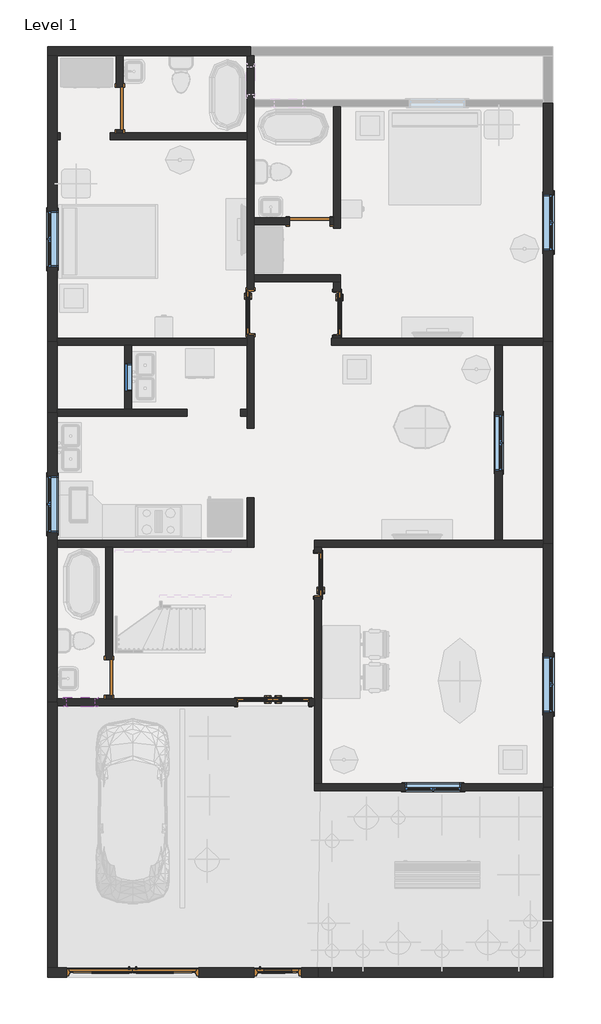
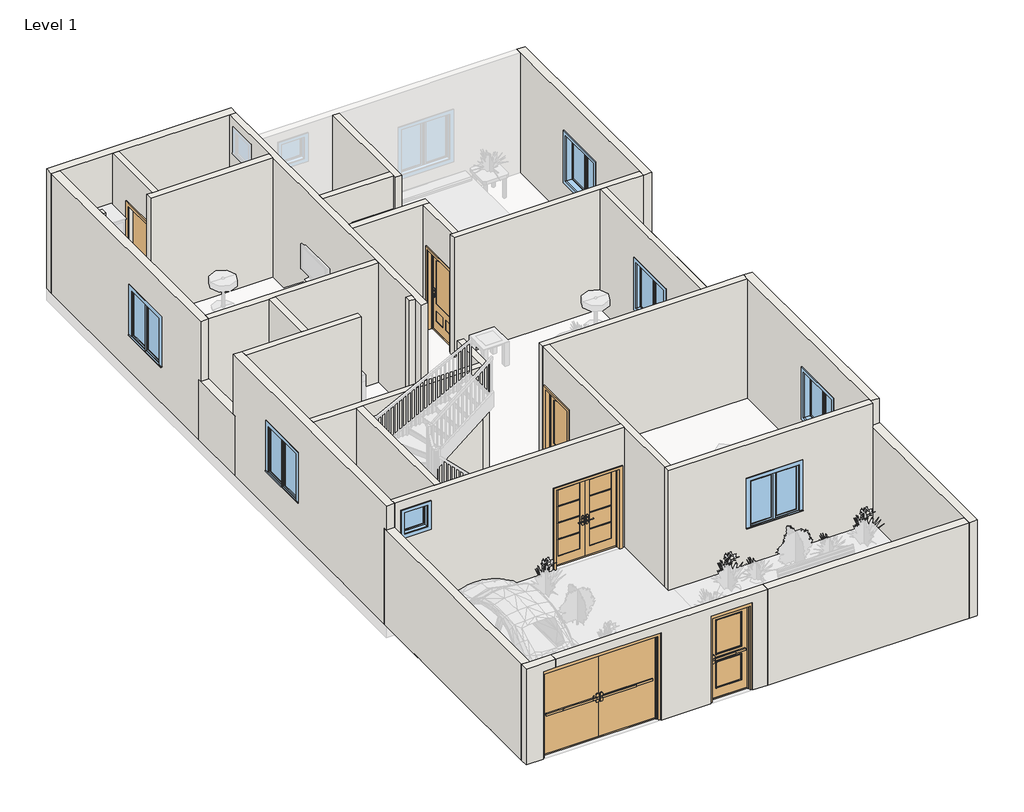
# One storey, part 1 of 3: 33 walls, 9 doors, 8 windows.
"""IFC4 building model written with IfcOpenShell, lengths in millimetres."""

from ifc_helpers import new_model, si_unit, frame, origin, origin_with_axes, place, context, project, spatial, polyline, outline, extrude, faceted_brep, transform, mapped, element, save
from components import door_808aeb8e, door_5d363d20, door_b5c84c7e, door_94998e6c, door_exterior_single_two_lite_door_exterior_single_two_lite_36a17ea7, door_059fdd7e, door_b6e9fca3, door_16372e1c, window_0862ab64, window_be30da88, window_aff1bc2a, window_3d781103

model = new_model("IFC4")

# Units and contexts
model_context = context("Model", 3, world=origin())
ifc_project = project(units=[si_unit("LENGTHUNIT", "METRE", prefix="MILLI")], contexts=[model_context])

# Site, building, storey
site = spatial("IfcSite", under=ifc_project)
building = spatial("IfcBuilding", under=site)
storey = spatial("IfcBuildingStorey", under=building, Name="Level 1", Elevation=0.0)

# Doors
placement = place(None, origin())
door_shape = door_808aeb8e(model_context)
element("IfcDoor", 1, ObjectType="36\" x 80\"", at=placement, inside=storey, context=model_context, shape_type="MappedRepresentation", body=[
    mapped(door_shape, transform((-7436.4726606, 8433.499435, 0.0), x_axis=(0.0, 1.0, 0.0), y_axis=(-1.0, 0.0, 0.0), z_axis=(0.0, 0.0, 1.0))),
])
element("IfcDoor", 2, ObjectType="36\" x 80\"", at=placement, inside=storey, context=model_context, shape_type="MappedRepresentation", body=[
    mapped(door_shape, transform((-5982.3226606, 2794.699435, 0.0), x_axis=(0.0, -1.0, 0.0), y_axis=(1.0, 0.0, 0.0), z_axis=(0.0, 0.0, 1.0))),
])
door_2_shape = door_5d363d20(model_context)
element("IfcDoor", 3, ObjectType="36\" x 80\"", at=placement, inside=storey, context=model_context, shape_type="MappedRepresentation", body=[
    mapped(door_2_shape, transform((-5575.9226606, 8408.099435, 0.0), x_axis=(0.0, 1.0, 0.0), y_axis=(-1.0, 0.0, 0.0), z_axis=(0.0, 0.0, 1.0))),
])
door_3_shape = door_b5c84c7e(model_context)
element("IfcDoor", 4, ObjectType="Door-Exterior-Double : 108\" x 84\"", at=placement, inside=storey, context=model_context, shape_type="MappedRepresentation", body=[
    mapped(door_3_shape, transform((-9973.2976606, -5771.450565, 0.0), x_axis=(1.0, 0.0, 0.0), y_axis=(0.0, 1.0, 0.0), z_axis=(0.0, 0.0, 1.0))),
])
door_4_shape = door_94998e6c(model_context)
element("IfcDoor", 5, ObjectType="Door-Exterior-Double-Full Glass-Wood_Clad : 60\" x 80\"", at=placement, inside=storey, context=model_context, shape_type="MappedRepresentation", body=[
    mapped(door_4_shape, transform((-6950.6976606, 54.674435, 0.0), x_axis=(1.0, 0.0, 0.0), y_axis=(0.0, 1.0, 0.0), z_axis=(0.0, 0.0, 1.0))),
])
door_exterior_single_two_lite_door_exterior_single_two_lite_shape = door_exterior_single_two_lite_door_exterior_single_two_lite_36a17ea7(model_context)
element("IfcDoor", 6, ObjectType="Door-Exterior-Single-Two_Lite : Door-Exterior-Single-Two_Lite", at=placement, inside=storey, context=model_context, shape_type="MappedRepresentation", body=[
    mapped(door_exterior_single_two_lite_door_exterior_single_two_lite_shape, transform((-6849.0976606, -5771.450565, 0.0), x_axis=(1.0, 0.0, 0.0), y_axis=(0.0, 1.0, 0.0), z_axis=(0.0, 0.0, 1.0))),
])
door_5_shape = door_059fdd7e(model_context)
element("IfcDoor", 7, ObjectType="Single-Flush : 30\" x 80\"", at=placement, inside=storey, context=model_context, shape_type="MappedRepresentation", body=[
    mapped(door_5_shape, transform((-10481.2976606, 584.899435, 0.0), x_axis=(0.0, -1.0, 0.0), y_axis=(1.0, 0.0, 0.0), z_axis=(0.0, 0.0, 1.0))),
])
door_6_shape = door_b6e9fca3(model_context)
element("IfcDoor", 8, ObjectType="Single-Flush : 34\" x 84\"", at=placement, inside=storey, context=model_context, shape_type="MappedRepresentation", body=[
    mapped(door_6_shape, transform((-6163.2976606, 10389.299435, 0.0), x_axis=(1.0, 0.0, 0.0), y_axis=(0.0, 1.0, 0.0), z_axis=(0.0, 0.0, 1.0))),
])
door_7_shape = door_16372e1c(model_context)
element("IfcDoor", 9, ObjectType="Single-Flush : 36\" x 84\"", at=placement, inside=storey, context=model_context, shape_type="MappedRepresentation", body=[
    mapped(door_7_shape, transform((-10252.6976606, 12814.999435, 0.0), x_axis=(0.0, -1.0, 0.0), y_axis=(1.0, 0.0, 0.0), z_axis=(0.0, 0.0, 1.0))),
])

# Walls
element("IfcWall", 10, at=placement, inside=storey, context=model_context, shape_type="SweptSolid", body=[
    extrude(outline(polyline([(-5985.4976606, -5663.500565), (-1134.0976606, -5663.500565), (-1134.0976606, -5866.700565), (-5985.4976606, -5866.700565), (-5985.4976606, -5663.500565)])), origin_with_axes(), (0.0, 0.0, 1.0), 2438.4),
])
element("IfcWall", 11, at=placement, inside=storey, context=model_context, shape_type="Brep", body=[
    faceted_brep([(-11598.8976606, -5663.500565, 0.0), (-11598.8976606, -24.700565, 0.0), (-11598.8976606, 51.499435, 0.0), (-11598.8976606, 51.499435, 2438.4), (-11598.8976606, -5663.500565, 2438.4), (-11802.0976606, -5663.500565, 0.0), (-11802.0976606, -5663.500565, 2438.4), (-11802.0976606, 51.499435, 2438.4), (-11802.0976606, 51.499435, 0.0)], [[[0, 1, 2, 3, 4]], [[5, 6, 7, 8]], [[2, 1, 0, 5, 8]], [[3, 2, 8, 7]], [[4, 3, 7, 6]], [[0, 4, 6, 5]]]),
])
element("IfcWall", 12, at=placement, inside=storey, context=model_context, shape_type="SweptSolid", body=[
    extrude(outline(polyline([(2438.4, -5985.4976606), (2438.4, -11090.8976606), (2235.2, -11090.8976606), (2235.2, -8550.8976606), (0.0, -8550.8976606), (0.0, -7357.0976606), (2235.2, -7357.0976606), (2235.2, -6341.0976606), (0.0, -6341.0976606), (0.0, -5985.4976606), (2438.4, -5985.4976606)])), frame((0.0, -5866.700565, 0.0), z_axis=(0.0, 1.0, 0.0), x_axis=(0.0, 0.0, 1.0)), (0.0, 0.0, 1.0), 203.2),
])
element("IfcWall", 13, at=placement, inside=storey, context=model_context, shape_type="Brep", body=[
    faceted_brep([(-1134.0976606, -1790.000565, 0.0), (-1134.0976606, -1853.500565, 0.0), (-1134.0976606, -5663.500565, 0.0), (-1134.0976606, -5866.700565, 0.0), (-1134.0976606, -5866.700565, 2438.4), (-1134.0976606, -5663.500565, 2438.4), (-1134.0976606, -1790.000565, 2438.4), (-930.8976606, -1790.000565, 0.0), (-930.8976606, -1790.000565, 2438.4), (-930.8976606, -5866.700565, 2438.4), (-930.8976606, -5866.700565, 0.0)], [[[0, 1, 2, 3, 4, 5, 6]], [[7, 8, 9, 10]], [[3, 2, 1, 0, 7, 10]], [[6, 5, 4, 9, 8]], [[0, 6, 8, 7]], [[4, 3, 10, 9]]]),
])
element("IfcWall", 14, at=placement, inside=storey, context=model_context, shape_type="Brep", body=[
    faceted_brep([(-11802.0976606, -5663.500565, 2438.4), (-11598.8976606, -5663.500565, 2438.4), (-11090.8976606, -5663.500565, 2438.4), (-11090.8976606, -5663.500565, 2235.2), (-11395.6976606, -5663.500565, 2235.2), (-11395.6976606, -5663.500565, 0.0), (-11598.8976606, -5663.500565, 0.0), (-11802.0976606, -5663.500565, 0.0), (-11090.8976606, -5866.700565, 2438.4), (-11802.0976606, -5866.700565, 2438.4), (-11802.0976606, -5866.700565, 0.0), (-11395.6976606, -5866.700565, 0.0), (-11395.6976606, -5866.700565, 2235.2), (-11090.8976606, -5866.700565, 2235.2)], [[[0, 1, 2, 3, 4, 5, 6, 7]], [[8, 9, 10, 11, 12, 13]], [[10, 7, 6, 5, 11]], [[2, 1, 0, 9, 8]], [[2, 8, 13, 3]], [[0, 7, 10, 9]], [[12, 4, 3, 13]], [[4, 12, 11, 5]]]),
])
element("IfcWall", 15, ObjectType="Generic - 8\"", at=placement, inside=storey, context=model_context, shape_type="Brep", body=[
    faceted_brep([(-11802.0976606, 13945.299435, 0.0), (-11598.8976606, 13945.299435, 0.0), (-10328.8976606, 13945.299435, 0.0), (-10176.4976606, 13945.299435, 0.0), (-7509.4976606, 13945.299435, 0.0), (-7433.2976606, 13945.299435, 0.0), (-7433.2976606, 13945.299435, 1524.0), (-7357.0976606, 13945.299435, 1524.0), (-7357.0976606, 13945.299435, 3048.0), (-7509.4976606, 13945.299435, 3048.0), (-10176.4976606, 13945.299435, 3048.0), (-10328.8976606, 13945.299435, 3048.0), (-11598.8976606, 13945.299435, 3048.0), (-11802.0976606, 13945.299435, 3048.0), (-11802.0976606, 14148.499435, 0.0), (-11802.0976606, 14148.499435, 3048.0), (-7357.0976606, 14148.499435, 3048.0), (-7357.0976606, 14148.499435, 1524.0), (-7433.2976606, 14148.499435, 1524.0), (-7433.2976606, 14148.499435, 0.0)], [[[0, 1, 2, 3, 4, 5, 6, 7, 8, 9, 10, 11, 12, 13]], [[14, 15, 16, 17, 18, 19]], [[5, 4, 3, 2, 1, 0, 14, 19]], [[0, 13, 15, 14]], [[6, 5, 19, 18]], [[17, 7, 6, 18]], [[8, 7, 17, 16]], [[13, 12, 11, 10, 9, 8, 16, 15]]]),
])
element("IfcWall", 16, ObjectType="Generic - 8\"", at=placement, inside=storey, context=model_context, shape_type="Brep", body=[
    faceted_brep([(-1134.0976606, 7798.499435, 0.0), (-1134.0976606, 7722.299435, 0.0), (-1134.0976606, 3531.299435, 0.0), (-1134.0976606, 3455.099435, 0.0), (-1134.0976606, 3455.099435, 1524.0), (-1134.0976606, 3531.299435, 1524.0), (-1134.0976606, 7722.299435, 1524.0), (-1134.0976606, 7798.499435, 1524.0), (-930.8976606, 7798.499435, 0.0), (-930.8976606, 7798.499435, 1524.0), (-930.8976606, 7722.299435, 1524.0), (-930.8976606, 3531.299435, 1524.0), (-930.8976606, 3455.099435, 1524.0), (-930.8976606, 3455.099435, 0.0)], [[[0, 1, 2, 3, 4, 5, 6, 7]], [[8, 9, 10, 11, 12, 13]], [[3, 2, 1, 0, 8, 13]], [[4, 3, 13, 12]], [[7, 6, 5, 4, 12, 11, 10, 9]], [[0, 7, 9, 8]]]),
])
element("IfcWall", 17, ObjectType="Generic - 8\"", at=placement, inside=storey, context=model_context, shape_type="Brep", body=[
    faceted_brep([(-1134.0976606, 3455.099435, 0.0), (-1134.0976606, 3378.899435, 0.0), (-1134.0976606, -1764.600565, 0.0), (-1134.0976606, -1764.600565, 3048.0), (-1134.0976606, 3378.899435, 3048.0), (-1134.0976606, 3531.299435, 3048.0), (-1134.0976606, 3531.299435, 1524.0), (-1134.0976606, 3455.099435, 1524.0), (-1134.0976606, -177.100565, 2133.6), (-1134.0976606, -177.100565, 914.4), (-1134.0976606, 1042.099435, 914.4), (-1134.0976606, 1042.099435, 2133.6), (-930.8976606, 3455.099435, 0.0), (-930.8976606, 3455.099435, 1524.0), (-930.8976606, 3531.299435, 1524.0), (-930.8976606, 3531.299435, 3048.0), (-930.8976606, -1764.600565, 3048.0), (-930.8976606, -1764.600565, 0.0), (-930.8976606, -177.100565, 2133.6), (-930.8976606, 1042.099435, 2133.6), (-930.8976606, 1042.099435, 914.4), (-930.8976606, -177.100565, 914.4)], [[[0, 1, 2, 3, 4, 5, 6, 7], [8, 9, 10, 11]], [[12, 13, 14, 15, 16, 17], [18, 19, 20, 21]], [[2, 1, 0, 12, 17]], [[3, 2, 17, 16]], [[0, 7, 13, 12]], [[6, 14, 13, 7]], [[6, 5, 15, 14]], [[9, 8, 18, 21]], [[10, 9, 21, 20]], [[11, 10, 20, 19]], [[8, 11, 19, 18]], [[5, 4, 3, 16, 15]]]),
])
element("IfcWall", 18, ObjectType="Generic - 8\"", at=placement, inside=storey, context=model_context, shape_type="Brep", body=[
    faceted_brep([(-1134.0976606, 12929.299435, 0.0), (-1134.0976606, 12853.099435, 0.0), (-1134.0976606, 7874.699435, 0.0), (-1134.0976606, 7798.499435, 0.0), (-1134.0976606, 7798.499435, 1524.0), (-1134.0976606, 7722.299435, 1524.0), (-1134.0976606, 7722.299435, 3048.0), (-1134.0976606, 7874.699435, 3048.0), (-1134.0976606, 12853.099435, 3048.0), (-1134.0976606, 13005.499435, 3048.0), (-1134.0976606, 13005.499435, 1524.0), (-1134.0976606, 12929.299435, 1524.0), (-1134.0976606, 9754.299435, 2133.6), (-1134.0976606, 9754.299435, 914.4), (-1134.0976606, 10973.499435, 914.4), (-1134.0976606, 10973.499435, 2133.6), (-930.8976606, 12929.299435, 0.0), (-930.8976606, 12929.299435, 1524.0), (-930.8976606, 13005.499435, 1524.0), (-930.8976606, 13005.499435, 3048.0), (-930.8976606, 7722.299435, 3048.0), (-930.8976606, 7722.299435, 1524.0), (-930.8976606, 7798.499435, 1524.0), (-930.8976606, 7798.499435, 0.0), (-930.8976606, 9754.299435, 2133.6), (-930.8976606, 10973.499435, 2133.6), (-930.8976606, 10973.499435, 914.4), (-930.8976606, 9754.299435, 914.4)], [[[0, 1, 2, 3, 4, 5, 6, 7, 8, 9, 10, 11], [12, 13, 14, 15]], [[16, 17, 18, 19, 20, 21, 22, 23], [24, 25, 26, 27]], [[3, 2, 1, 0, 16, 23]], [[4, 3, 23, 22]], [[21, 5, 4, 22]], [[6, 5, 21, 20]], [[0, 11, 17, 16]], [[10, 18, 17, 11]], [[10, 9, 19, 18]], [[13, 12, 24, 27]], [[14, 13, 27, 26]], [[15, 14, 26, 25]], [[12, 15, 25, 24]], [[9, 8, 7, 6, 20, 19]]]),
])
element("IfcWall", 19, ObjectType="Generic - 8\"", at=placement, inside=storey, context=model_context, shape_type="Brep", body=[
    faceted_brep([(-11598.8976606, 7798.499435, 0.0), (-11598.8976606, 7874.699435, 0.0), (-11598.8976606, 12141.899435, 0.0), (-11598.8976606, 12294.299435, 0.0), (-11598.8976606, 13945.299435, 0.0), (-11598.8976606, 13945.299435, 3048.0), (-11598.8976606, 12294.299435, 3048.0), (-11598.8976606, 12141.899435, 3048.0), (-11598.8976606, 7874.699435, 3048.0), (-11598.8976606, 7722.299435, 3048.0), (-11598.8976606, 7722.299435, 1524.0), (-11598.8976606, 7798.499435, 1524.0), (-11598.8976606, 10617.899435, 2133.6), (-11598.8976606, 10617.899435, 914.4), (-11598.8976606, 9398.699435, 914.4), (-11598.8976606, 9398.699435, 2133.6), (-11802.0976606, 7798.499435, 0.0), (-11802.0976606, 7798.499435, 1524.0), (-11802.0976606, 7722.299435, 1524.0), (-11802.0976606, 7722.299435, 3048.0), (-11802.0976606, 13945.299435, 3048.0), (-11802.0976606, 13945.299435, 0.0), (-11802.0976606, 10617.899435, 2133.6), (-11802.0976606, 9398.699435, 2133.6), (-11802.0976606, 9398.699435, 914.4), (-11802.0976606, 10617.899435, 914.4)], [[[0, 1, 2, 3, 4, 5, 6, 7, 8, 9, 10, 11], [12, 13, 14, 15]], [[16, 17, 18, 19, 20, 21], [22, 23, 24, 25]], [[4, 3, 2, 1, 0, 16, 21]], [[5, 4, 21, 20]], [[13, 12, 22, 25]], [[14, 13, 25, 24]], [[15, 14, 24, 23]], [[12, 15, 23, 22]], [[0, 11, 17, 16]], [[10, 18, 17, 11]], [[10, 9, 19, 18]], [[9, 8, 7, 6, 5, 20, 19]]]),
])
element("IfcWall", 20, ObjectType="Generic - 8\"", at=placement, inside=storey, context=model_context, shape_type="Brep", body=[
    faceted_brep([(-11598.8976606, 6274.499435, 0.0), (-11598.8976606, 6350.699435, 0.0), (-11598.8976606, 7722.299435, 0.0), (-11598.8976606, 7798.499435, 0.0), (-11598.8976606, 7798.499435, 1524.0), (-11598.8976606, 7722.299435, 1524.0), (-11598.8976606, 6350.699435, 1524.0), (-11598.8976606, 6274.499435, 1524.0), (-11802.0976606, 6274.499435, 0.0), (-11802.0976606, 6274.499435, 1524.0), (-11802.0976606, 6350.699435, 1524.0), (-11802.0976606, 7722.299435, 1524.0), (-11802.0976606, 7798.499435, 1524.0), (-11802.0976606, 7798.499435, 0.0)], [[[0, 1, 2, 3, 4, 5, 6, 7]], [[8, 9, 10, 11, 12, 13]], [[3, 2, 1, 0, 8, 13]], [[4, 3, 13, 12]], [[7, 6, 5, 4, 12, 11, 10, 9]], [[0, 7, 9, 8]]]),
])
element("IfcWall", 21, ObjectType="Generic - 8\"", at=placement, inside=storey, context=model_context, shape_type="Brep", body=[
    faceted_brep([(-11598.8976606, 51.499435, 0.0), (-11598.8976606, 127.699435, 0.0), (-11598.8976606, 3378.899435, 0.0), (-11598.8976606, 3531.299435, 0.0), (-11598.8976606, 6198.299435, 0.0), (-11598.8976606, 6274.499435, 0.0), (-11598.8976606, 6274.499435, 1524.0), (-11598.8976606, 6350.699435, 1524.0), (-11598.8976606, 6350.699435, 3048.0), (-11598.8976606, 6198.299435, 3048.0), (-11598.8976606, 3531.299435, 3048.0), (-11598.8976606, 3378.899435, 3048.0), (-11598.8976606, 127.699435, 3048.0), (-11598.8976606, -24.700565, 3048.0), (-11598.8976606, -24.700565, 2438.4), (-11598.8976606, 51.499435, 2438.4), (-11598.8976606, 4915.599435, 2133.6), (-11598.8976606, 4915.599435, 914.4), (-11598.8976606, 3696.399435, 914.4), (-11598.8976606, 3696.399435, 2133.6), (-11802.0976606, 51.499435, 0.0), (-11802.0976606, 51.499435, 2438.4), (-11802.0976606, -24.700565, 2438.4), (-11802.0976606, -24.700565, 3048.0), (-11802.0976606, 6350.699435, 3048.0), (-11802.0976606, 6350.699435, 1524.0), (-11802.0976606, 6274.499435, 1524.0), (-11802.0976606, 6274.499435, 0.0), (-11802.0976606, 4915.599435, 2133.6), (-11802.0976606, 3696.399435, 2133.6), (-11802.0976606, 3696.399435, 914.4), (-11802.0976606, 4915.599435, 914.4)], [[[0, 1, 2, 3, 4, 5, 6, 7, 8, 9, 10, 11, 12, 13, 14, 15], [16, 17, 18, 19]], [[20, 21, 22, 23, 24, 25, 26, 27], [28, 29, 30, 31]], [[5, 4, 3, 2, 1, 0, 20, 27]], [[6, 5, 27, 26]], [[25, 7, 6, 26]], [[8, 7, 25, 24]], [[16, 19, 29, 28]], [[19, 18, 30, 29]], [[18, 17, 31, 30]], [[17, 16, 28, 31]], [[0, 15, 21, 20]], [[14, 22, 21, 15]], [[14, 13, 23, 22]], [[13, 12, 11, 10, 9, 8, 24, 23]]]),
])
element("IfcWall", 22, ObjectType="INNER 6\"", at=placement, inside=storey, context=model_context, shape_type="SweptSolid", body=[
    extrude(outline(polyline([(-11535.3976606, 12141.899435), (-11598.8976606, 12141.899435), (-11598.8976606, 12294.299435), (-11535.3976606, 12294.299435), (-11535.3976606, 12141.899435)])), origin_with_axes(), (0.0, 0.0, 1.0), 3048.0),
])
element("IfcWall", 23, ObjectType="INNER 6\"", at=placement, inside=storey, context=model_context, shape_type="Brep", body=[
    faceted_brep([(-1134.0976606, 7874.699435, 3048.0), (-1134.0976606, 7874.699435, 0.0), (-5502.8976606, 7874.699435, 0.0), (-5655.2976606, 7874.699435, 0.0), (-5693.3976606, 7874.699435, 0.0), (-5693.3976606, 7874.699435, 3048.0), (-5655.2976606, 7874.699435, 3048.0), (-5502.8976606, 7874.699435, 3048.0), (-1134.0976606, 7722.299435, 0.0), (-1134.0976606, 7722.299435, 1524.0), (-1134.0976606, 7722.299435, 3048.0), (-2023.0976606, 7722.299435, 3048.0), (-2175.4976606, 7722.299435, 3048.0), (-5693.3976606, 7722.299435, 3048.0), (-5693.3976606, 7722.299435, 0.0), (-2175.4976606, 7722.299435, 0.0), (-2023.0976606, 7722.299435, 0.0), (-1134.0976606, 7798.499435, 0.0)], [[[0, 1, 2, 3, 4, 5, 6, 7]], [[8, 9, 10, 11, 12, 13, 14, 15, 16]], [[4, 3, 2, 1, 17, 8, 16, 15, 14]], [[5, 4, 14, 13]], [[0, 10, 9, 8, 17, 1]], [[0, 7, 6, 5, 13, 12, 11, 10]]]),
])
element("IfcWall", 24, ObjectType="INNER 6\"", at=placement, inside=storey, context=model_context, shape_type="Brep", body=[
    faceted_brep([(-5655.2976606, 12853.099435, 0.0), (-5655.2976606, 10465.499435, 0.0), (-5655.2976606, 10313.099435, 0.0), (-5655.2976606, 10236.899435, 0.0), (-5655.2976606, 10236.899435, 3048.0), (-5655.2976606, 10313.099435, 3048.0), (-5655.2976606, 10465.499435, 3048.0), (-5655.2976606, 12853.099435, 3048.0), (-5502.8976606, 12853.099435, 0.0), (-5502.8976606, 12853.099435, 3048.0), (-5502.8976606, 10236.899435, 3048.0), (-5502.8976606, 10236.899435, 0.0)], [[[0, 1, 2, 3, 4, 5, 6, 7]], [[8, 9, 10, 11]], [[3, 2, 1, 0, 8, 11]], [[4, 3, 11, 10]], [[0, 7, 9, 8]], [[7, 6, 5, 4, 10, 9]]]),
])
element("IfcWall", 25, ObjectType="INNER 6\"", at=placement, inside=storey, context=model_context, shape_type="SweptSolid", body=[
    extrude(outline(polyline([(2133.6, -5731.4976606), (0.0, -5731.4976606), (0.0, -5655.2976606), (3048.0, -5655.2976606), (3048.0, -7357.0976606), (0.0, -7357.0976606), (0.0, -6595.0976606), (2133.6, -6595.0976606), (2133.6, -5731.4976606)])), frame((0.0, 10313.099435, 0.0), z_axis=(0.0, 1.0, 0.0), x_axis=(0.0, 0.0, 1.0)), (0.0, 0.0, 1.0), 152.4),
])
element("IfcWall", 26, ObjectType="INNER 6\"", at=placement, inside=storey, context=model_context, shape_type="Brep", body=[
    faceted_brep([(-5502.8976606, 9246.299435, 0.0), (-7357.0976606, 9246.299435, 0.0), (-7357.0976606, 9246.299435, 3048.0), (-5502.8976606, 9246.299435, 3048.0), (-5502.8976606, 9093.899435, 0.0), (-5502.8976606, 9093.899435, 3048.0), (-5655.2976606, 9093.899435, 3048.0), (-7357.0976606, 9093.899435, 3048.0), (-7357.0976606, 9093.899435, 0.0), (-5655.2976606, 9093.899435, 0.0)], [[[0, 1, 2, 3]], [[4, 5, 6, 7, 8, 9]], [[1, 0, 4, 9, 8]], [[2, 1, 8, 7]], [[0, 3, 5, 4]], [[3, 2, 7, 6, 5]]]),
])
element("IfcWall", 27, ObjectType="INNER 6\"", at=placement, inside=storey, context=model_context, shape_type="Brep", body=[
    faceted_brep([(-7357.0976606, 3378.899435, 0.0), (-7357.0976606, 4445.699435, 0.0), (-7357.0976606, 4445.699435, 3048.0), (-7357.0976606, 3378.899435, 3048.0), (-7509.4976606, 3378.899435, 0.0), (-7509.4976606, 3378.899435, 3048.0), (-7509.4976606, 3531.299435, 3048.0), (-7509.4976606, 4445.699435, 3048.0), (-7509.4976606, 4445.699435, 0.0), (-7509.4976606, 3531.299435, 0.0)], [[[0, 1, 2, 3]], [[4, 5, 6, 7, 8, 9]], [[1, 0, 4, 9, 8]], [[2, 1, 8, 7]], [[0, 3, 5, 4]], [[3, 2, 7, 6, 5]]]),
])
element("IfcWall", 28, ObjectType="INNER 6\"", at=placement, inside=storey, context=model_context, shape_type="Brep", body=[
    faceted_brep([(-11598.8976606, 6198.299435, 3048.0), (-11598.8976606, 6198.299435, 0.0), (-8804.8976606, 6198.299435, 0.0), (-8804.8976606, 6198.299435, 3048.0), (-11598.8976606, 6350.699435, 0.0), (-11598.8976606, 6350.699435, 1524.0), (-11598.8976606, 6350.699435, 3048.0), (-10151.0976606, 6350.699435, 3048.0), (-9998.6976606, 6350.699435, 3048.0), (-8804.8976606, 6350.699435, 3048.0), (-8804.8976606, 6350.699435, 0.0), (-9998.6976606, 6350.699435, 0.0), (-10151.0976606, 6350.699435, 0.0), (-11598.8976606, 6274.499435, 0.0)], [[[0, 1, 2, 3]], [[4, 5, 6, 7, 8, 9, 10, 11, 12]], [[2, 1, 13, 4, 12, 11, 10]], [[3, 2, 10, 9]], [[0, 6, 5, 4, 13, 1]], [[0, 3, 9, 8, 7, 6]]]),
])
element("IfcWall", 29, ObjectType="INNER 6\"", at=placement, inside=storey, context=model_context, shape_type="SweptSolid", body=[
    extrude(outline(polyline([(6350.699435, 0.0), (6350.699435, 3048.0), (7722.299435, 3048.0), (7722.299435, 0.0), (6350.699435, 0.0)]), holes=[polyline([(7341.299435, 1752.6), (6731.699435, 1752.6), (6731.699435, 1143.0), (7341.299435, 1143.0), (7341.299435, 1752.6)])]), frame((-10151.0976606, 0.0, 0.0), z_axis=(1.0, 0.0, 0.0), x_axis=(0.0, 1.0, 0.0)), (0.0, 0.0, 1.0), 152.4),
])
element("IfcWall", 30, ObjectType="INNER 6\"", at=placement, inside=storey, context=model_context, shape_type="Brep", body=[
    faceted_brep([(-11598.8976606, 3378.899435, 0.0), (-10557.4976606, 3378.899435, 0.0), (-10405.0976606, 3378.899435, 0.0), (-7509.4976606, 3378.899435, 0.0), (-7509.4976606, 3378.899435, 3048.0), (-10405.0976606, 3378.899435, 3048.0), (-10557.4976606, 3378.899435, 3048.0), (-11598.8976606, 3378.899435, 3048.0), (-11598.8976606, 3531.299435, 0.0), (-11598.8976606, 3531.299435, 3048.0), (-7509.4976606, 3531.299435, 3048.0), (-7509.4976606, 3531.299435, 0.0)], [[[0, 1, 2, 3, 4, 5, 6, 7]], [[8, 9, 10, 11]], [[3, 2, 1, 0, 8, 11]], [[0, 7, 9, 8]], [[4, 3, 11, 10]], [[7, 6, 5, 4, 10, 9]]]),
])
element("IfcWall", 31, ObjectType="INNER 6\"", at=placement, inside=storey, context=model_context, shape_type="Brep", body=[
    faceted_brep([(-6061.6976606, -24.700565, 0.0), (-6061.6976606, -24.700565, 3048.0), (-11598.8976606, -24.700565, 3048.0), (-11598.8976606, -24.700565, 2438.4), (-11598.8976606, -24.700565, 0.0), (-7738.0976606, -24.700565, 0.0), (-7738.0976606, -24.700565, 2057.4), (-6163.2976606, -24.700565, 2057.4), (-6163.2976606, -24.700565, 0.0), (-10786.0976606, -24.700565, 2768.6), (-10786.0976606, -24.700565, 2159.0), (-11395.6976606, -24.700565, 2159.0), (-11395.6976606, -24.700565, 2768.6), (-6061.6976606, 127.699435, 3048.0), (-6061.6976606, 127.699435, 0.0), (-6163.2976606, 127.699435, 0.0), (-6163.2976606, 127.699435, 2057.4), (-7738.0976606, 127.699435, 2057.4), (-7738.0976606, 127.699435, 0.0), (-10405.0976606, 127.699435, 0.0), (-10557.4976606, 127.699435, 0.0), (-11598.8976606, 127.699435, 0.0), (-11598.8976606, 127.699435, 3048.0), (-10557.4976606, 127.699435, 3048.0), (-10405.0976606, 127.699435, 3048.0), (-10786.0976606, 127.699435, 2768.6), (-11395.6976606, 127.699435, 2768.6), (-11395.6976606, 127.699435, 2159.0), (-10786.0976606, 127.699435, 2159.0), (-11598.8976606, 51.499435, 0.0)], [[[0, 1, 2, 3, 4, 5, 6, 7, 8], [9, 10, 11, 12]], [[13, 14, 15, 16, 17, 18, 19, 20, 21, 22, 23, 24], [25, 26, 27, 28]], [[14, 0, 8, 15]], [[4, 29, 21, 20, 19, 18, 5]], [[1, 0, 14, 13]], [[7, 16, 15, 8]], [[16, 7, 6, 17]], [[17, 6, 5, 18]], [[10, 9, 25, 28]], [[11, 10, 28, 27]], [[12, 11, 27, 26]], [[9, 12, 26, 25]], [[21, 29, 4, 3, 2, 22]], [[2, 1, 13, 24, 23, 22]]]),
])
element("IfcWall", 32, ObjectType="INNER 6\"", at=placement, inside=storey, context=model_context, shape_type="SweptSolid", body=[
    extrude(outline(polyline([(203.899435, 2032.0), (203.899435, 0.0), (127.699435, 0.0), (127.699435, 3048.0), (3378.899435, 3048.0), (3378.899435, 0.0), (965.899435, 0.0), (965.899435, 2032.0), (203.899435, 2032.0)])), frame((-10557.4976606, 0.0, 0.0), z_axis=(1.0, 0.0, 0.0), x_axis=(0.0, 1.0, 0.0)), (0.0, 0.0, 1.0), 152.4),
])
element("IfcWall", 33, ObjectType="INNER 6\"", at=placement, inside=storey, context=model_context, shape_type="Brep", body=[
    faceted_brep([(-5909.2976606, 3378.899435, 0.0), (-5909.2976606, 3378.899435, 3048.0), (-5909.2976606, -1701.100565, 3048.0), (-5909.2976606, -1701.100565, 0.0), (-5909.2976606, 2312.099435, 0.0), (-5909.2976606, 2312.099435, 2057.4), (-5909.2976606, 3277.299435, 2057.4), (-5909.2976606, 3277.299435, 0.0), (-6061.6976606, 3378.899435, 3048.0), (-6061.6976606, 3378.899435, 0.0), (-6061.6976606, 3277.299435, 0.0), (-6061.6976606, 3277.299435, 2057.4), (-6061.6976606, 2312.099435, 2057.4), (-6061.6976606, 2312.099435, 0.0), (-6061.6976606, 127.699435, 0.0), (-6061.6976606, -24.700565, 0.0), (-6061.6976606, -1701.100565, 0.0), (-6061.6976606, -1701.100565, 3048.0), (-6061.6976606, -24.700565, 3048.0), (-6061.6976606, 127.699435, 3048.0)], [[[0, 1, 2, 3, 4, 5, 6, 7]], [[8, 9, 10, 11, 12, 13, 14, 15, 16, 17, 18, 19]], [[9, 0, 7, 10]], [[3, 16, 15, 14, 13, 4]], [[1, 0, 9, 8]], [[3, 2, 17, 16]], [[12, 5, 4, 13]], [[5, 12, 11, 6]], [[6, 11, 10, 7]], [[17, 2, 1, 8, 19, 18]]]),
])
element("IfcWall", 34, ObjectType="INNER 6\"", at=placement, inside=storey, context=model_context, shape_type="Brep", body=[
    faceted_brep([(-1134.0976606, 3531.299435, 3048.0), (-1134.0976606, 3531.299435, 1524.0), (-1134.0976606, 3531.299435, 0.0), (-2023.0976606, 3531.299435, 0.0), (-2175.4976606, 3531.299435, 0.0), (-6061.6976606, 3531.299435, 0.0), (-6061.6976606, 3531.299435, 3048.0), (-2175.4976606, 3531.299435, 3048.0), (-2023.0976606, 3531.299435, 3048.0), (-1134.0976606, 3378.899435, 0.0), (-1134.0976606, 3378.899435, 3048.0), (-5909.2976606, 3378.899435, 3048.0), (-6061.6976606, 3378.899435, 3048.0), (-6061.6976606, 3378.899435, 0.0), (-5909.2976606, 3378.899435, 0.0), (-1134.0976606, 3455.099435, 0.0)], [[[0, 1, 2, 3, 4, 5, 6, 7, 8]], [[9, 10, 11, 12, 13, 14]], [[5, 4, 3, 2, 15, 9, 14, 13]], [[0, 10, 9, 15, 2, 1]], [[6, 5, 13, 12]], [[0, 8, 7, 6, 12, 11, 10]]]),
])
element("IfcWall", 35, ObjectType="INNER 6\"", at=placement, inside=storey, context=model_context, shape_type="SweptSolid", body=[
    extrude(outline(polyline([(3531.299435, 0.0), (3531.299435, 3048.0), (7722.299435, 3048.0), (7722.299435, 0.0), (3531.299435, 0.0)]), holes=[polyline([(5017.199435, 2133.6), (5017.199435, 914.4), (6236.399435, 914.4), (6236.399435, 2133.6), (5017.199435, 2133.6)])]), frame((-2175.4976606, 0.0, 0.0), z_axis=(1.0, 0.0, 0.0), x_axis=(0.0, 1.0, 0.0)), (0.0, 0.0, 1.0), 152.4),
])
element("IfcWall", 36, ObjectType="INNER 6\"", at=placement, inside=storey, context=model_context, shape_type="Brep", body=[
    faceted_brep([(-1134.0976606, -1701.100565, 0.0), (-5909.2976606, -1701.100565, 0.0), (-6061.6976606, -1701.100565, 0.0), (-6061.6976606, -1701.100565, 3048.0), (-5909.2976606, -1701.100565, 3048.0), (-1134.0976606, -1701.100565, 3048.0), (-4118.5976606, -1701.100565, 2133.6), (-4118.5976606, -1701.100565, 914.4), (-2899.3976606, -1701.100565, 914.4), (-2899.3976606, -1701.100565, 2133.6), (-1134.0976606, -1853.500565, 0.0), (-1134.0976606, -1853.500565, 3048.0), (-6061.6976606, -1853.500565, 3048.0), (-6061.6976606, -1853.500565, 0.0), (-4118.5976606, -1853.500565, 2133.6), (-2899.3976606, -1853.500565, 2133.6), (-2899.3976606, -1853.500565, 914.4), (-4118.5976606, -1853.500565, 914.4), (-1134.0976606, -1790.000565, 0.0)], [[[0, 1, 2, 3, 4, 5], [6, 7, 8, 9]], [[10, 11, 12, 13], [14, 15, 16, 17]], [[2, 1, 0, 18, 10, 13]], [[0, 5, 11, 10, 18]], [[3, 2, 13, 12]], [[7, 6, 14, 17]], [[8, 7, 17, 16]], [[9, 8, 16, 15]], [[6, 9, 15, 14]], [[5, 4, 3, 12, 11]]]),
])
element("IfcWall", 37, ObjectType="INNER 6\"", at=placement, inside=storey, context=model_context, shape_type="SweptSolid", body=[
    extrude(outline(polyline([(12357.799435, 2133.6), (12357.799435, 0.0), (12294.299435, 0.0), (12294.299435, 3048.0), (13945.299435, 3048.0), (13945.299435, 0.0), (13272.199435, 0.0), (13272.199435, 2133.6), (12357.799435, 2133.6)])), frame((-10328.8976606, 0.0, 0.0), z_axis=(1.0, 0.0, 0.0), x_axis=(0.0, 1.0, 0.0)), (0.0, 0.0, 1.0), 152.4),
])
element("IfcWall", 38, ObjectType="INNER 6\"", at=placement, inside=storey, context=model_context, shape_type="Brep", body=[
    faceted_brep([(-10455.8976606, 12141.899435, 0.0), (-7509.4976606, 12141.899435, 0.0), (-7509.4976606, 12141.899435, 3048.0), (-10455.8976606, 12141.899435, 3048.0), (-10455.8976606, 12294.299435, 0.0), (-10455.8976606, 12294.299435, 3048.0), (-10328.8976606, 12294.299435, 3048.0), (-10176.4976606, 12294.299435, 3048.0), (-7509.4976606, 12294.299435, 3048.0), (-7509.4976606, 12294.299435, 0.0), (-10176.4976606, 12294.299435, 0.0), (-10328.8976606, 12294.299435, 0.0)], [[[0, 1, 2, 3]], [[4, 5, 6, 7, 8, 9, 10, 11]], [[1, 0, 4, 11, 10, 9]], [[0, 3, 5, 4]], [[2, 1, 9, 8]], [[3, 2, 8, 7, 6, 5]]]),
])
element("IfcWall", 39, ObjectType="INNER 6\"", at=placement, inside=storey, context=model_context, shape_type="Brep", body=[
    faceted_brep([(-7509.4976606, 7874.699435, 0.0), (-11598.8976606, 7874.699435, 0.0), (-11598.8976606, 7874.699435, 3048.0), (-7509.4976606, 7874.699435, 3048.0), (-7509.4976606, 7722.299435, 0.0), (-7509.4976606, 7722.299435, 3048.0), (-9998.6976606, 7722.299435, 3048.0), (-10151.0976606, 7722.299435, 3048.0), (-11598.8976606, 7722.299435, 3048.0), (-11598.8976606, 7722.299435, 1524.0), (-11598.8976606, 7722.299435, 0.0), (-10151.0976606, 7722.299435, 0.0), (-9998.6976606, 7722.299435, 0.0), (-11598.8976606, 7798.499435, 0.0)], [[[0, 1, 2, 3]], [[4, 5, 6, 7, 8, 9, 10, 11, 12]], [[1, 0, 4, 12, 11, 10, 13]], [[0, 3, 5, 4]], [[1, 13, 10, 9, 8, 2]], [[3, 2, 8, 7, 6, 5]]]),
])
element("IfcWall", 40, ObjectType="INNER 6\"", at=placement, inside=storey, context=model_context, shape_type="SweptSolid", body=[
    extrude(outline(polyline([(9093.899435, 3048.0), (9093.899435, 0.0), (8890.699435, 0.0), (8890.699435, 2057.4), (7925.499435, 2057.4), (7925.499435, 0.0), (7874.699435, 0.0), (7874.699435, 3048.0), (9093.899435, 3048.0)])), frame((-5655.2976606, 0.0, 0.0), z_axis=(1.0, 0.0, 0.0), x_axis=(0.0, 1.0, 0.0)), (0.0, 0.0, 1.0), 152.4),
])
element("IfcWall", 41, ObjectType="INNER 6\"", at=placement, inside=storey, context=model_context, shape_type="Brep", body=[
    faceted_brep([(-7357.0976606, 5944.299435, 3048.0), (-7357.0976606, 5944.299435, 0.0), (-7357.0976606, 7950.899435, 0.0), (-7357.0976606, 7950.899435, 2057.4), (-7357.0976606, 8916.099435, 2057.4), (-7357.0976606, 8916.099435, 0.0), (-7357.0976606, 9093.899435, 0.0), (-7357.0976606, 9246.299435, 0.0), (-7357.0976606, 10313.099435, 0.0), (-7357.0976606, 10465.499435, 0.0), (-7357.0976606, 12853.099435, 0.0), (-7357.0976606, 13005.499435, 0.0), (-7357.0976606, 13945.299435, 0.0), (-7357.0976606, 13945.299435, 1524.0), (-7357.0976606, 13945.299435, 3048.0), (-7357.0976606, 13005.499435, 3048.0), (-7357.0976606, 12853.099435, 3048.0), (-7357.0976606, 10465.499435, 3048.0), (-7357.0976606, 10313.099435, 3048.0), (-7357.0976606, 9246.299435, 3048.0), (-7357.0976606, 9093.899435, 3048.0), (-7357.0976606, 13716.699435, 2768.6), (-7357.0976606, 13716.699435, 2159.0), (-7357.0976606, 13107.099435, 2159.0), (-7357.0976606, 13107.099435, 2768.6), (-7509.4976606, 5944.299435, 0.0), (-7509.4976606, 5944.299435, 3048.0), (-7509.4976606, 6198.299435, 3048.0), (-7509.4976606, 6350.699435, 3048.0), (-7509.4976606, 7722.299435, 3048.0), (-7509.4976606, 7874.699435, 3048.0), (-7509.4976606, 12141.899435, 3048.0), (-7509.4976606, 12294.299435, 3048.0), (-7509.4976606, 13945.299435, 3048.0), (-7509.4976606, 13945.299435, 0.0), (-7509.4976606, 12294.299435, 0.0), (-7509.4976606, 12141.899435, 0.0), (-7509.4976606, 8916.099435, 0.0), (-7509.4976606, 8916.099435, 2057.4), (-7509.4976606, 7950.899435, 2057.4), (-7509.4976606, 7950.899435, 0.0), (-7509.4976606, 7874.699435, 0.0), (-7509.4976606, 7722.299435, 0.0), (-7509.4976606, 6350.699435, 0.0), (-7509.4976606, 6198.299435, 0.0), (-7509.4976606, 13716.699435, 2768.6), (-7509.4976606, 13107.099435, 2768.6), (-7509.4976606, 13107.099435, 2159.0), (-7509.4976606, 13716.699435, 2159.0), (-7433.2976606, 13945.299435, 0.0)], [[[0, 1, 2, 3, 4, 5, 6, 7, 8, 9, 10, 11, 12, 13, 14, 15, 16, 17, 18, 19, 20], [21, 22, 23, 24]], [[25, 26, 27, 28, 29, 30, 31, 32, 33, 34, 35, 36, 37, 38, 39, 40, 41, 42, 43, 44], [45, 46, 47, 48]], [[1, 25, 44, 43, 42, 41, 40, 2]], [[34, 49, 12, 11, 10, 9, 8, 7, 6, 5, 37, 36, 35]], [[1, 0, 26, 25]], [[4, 38, 37, 5]], [[38, 4, 3, 39]], [[39, 3, 2, 40]], [[12, 49, 34, 33, 14, 13]], [[22, 21, 45, 48]], [[23, 22, 48, 47]], [[24, 23, 47, 46]], [[21, 24, 46, 45]], [[0, 20, 19, 18, 17, 16, 15, 14, 33, 32, 31, 30, 29, 28, 27, 26]]]),
])
element("IfcWall", 42, ObjectType="INNER 6\"", at=placement, inside=storey, context=model_context, shape_type="SweptSolid", body=[
    extrude(outline(polyline([(-7509.4976606, 6198.299435), (-7649.1976606, 6198.299435), (-7649.1976606, 6350.699435), (-7509.4976606, 6350.699435), (-7509.4976606, 6198.299435)])), origin_with_axes(), (0.0, 0.0, 1.0), 3048.0),
])

# Windows
window_shape = window_0862ab64(model_context)
element("IfcWindow", 43, ObjectType="Casement Dbl with Trim : 48\" x 48\"", at=placement, inside=storey, context=model_context, shape_type="MappedRepresentation", body=[
    mapped(window_shape, transform((-11681.4476606, 10008.299435, 0.0), x_axis=(0.0, 1.0, 0.0), y_axis=(-1.0, 0.0, 0.0), z_axis=(0.0, 0.0, 1.0))),
])
element("IfcWindow", 44, ObjectType="Casement Dbl with Trim : 48\" x 48\"", at=placement, inside=storey, context=model_context, shape_type="MappedRepresentation", body=[
    mapped(window_shape, transform((-1051.5476606, 10363.899435, 0.0), x_axis=(0.0, -1.0, 0.0), y_axis=(1.0, 0.0, 0.0), z_axis=(0.0, 0.0, 1.0))),
])
element("IfcWindow", 45, ObjectType="Casement Dbl with Trim : 48\" x 48\"", at=placement, inside=storey, context=model_context, shape_type="MappedRepresentation", body=[
    mapped(window_shape, transform((-11681.4476606, 4305.999435, 0.0), x_axis=(0.0, 1.0, 0.0), y_axis=(-1.0, 0.0, 0.0), z_axis=(0.0, 0.0, 1.0))),
])
element("IfcWindow", 46, ObjectType="Casement Dbl with Trim : 48\" x 48\"", at=placement, inside=storey, context=model_context, shape_type="MappedRepresentation", body=[
    mapped(window_shape, transform((-1051.5476606, 432.499435, 0.0), x_axis=(0.0, -1.0, 0.0), y_axis=(1.0, 0.0, 0.0), z_axis=(0.0, 0.0, 1.0))),
])
window_2_shape = window_be30da88(model_context)
element("IfcWindow", 47, ObjectType="Casement Dbl with Trim : 48\" x 48\"", at=placement, inside=storey, context=model_context, shape_type="MappedRepresentation", body=[
    mapped(window_2_shape, transform((-3508.9976606, -1758.250565, 0.0), x_axis=(-1.0, 0.0, 0.0), y_axis=(0.0, -1.0, 0.0), z_axis=(0.0, 0.0, 1.0))),
])
element("IfcWindow", 48, ObjectType="Casement Dbl with Trim : 48\" x 48\"", at=placement, inside=storey, context=model_context, shape_type="MappedRepresentation", body=[
    mapped(window_2_shape, transform((-2118.3476606, 5626.799435, 0.0), x_axis=(0.0, -1.0, 0.0), y_axis=(1.0, 0.0, 0.0), z_axis=(0.0, 0.0, 1.0))),
])
window_3_shape = window_aff1bc2a(model_context)
element("IfcWindow", 49, ObjectType="Fixed : 24\" x 24\"", at=placement, inside=storey, context=model_context, shape_type="MappedRepresentation", body=[
    mapped(window_3_shape, transform((-10074.8976606, 7074.599435, 228.6), x_axis=(0.0, 1.0, 0.0), y_axis=(-1.0, 0.0, 0.0), z_axis=(0.0, 0.0, 1.0))),
])
window_4_shape = window_3d781103(model_context)
element("IfcWindow", 50, ObjectType="Transom with Trim : 24\" x 24\"", at=placement, inside=storey, context=model_context, shape_type="MappedRepresentation", body=[
    mapped(window_4_shape, transform((-11052.7976606, 51.499435, 0.0), x_axis=(1.0, 0.0, 0.0), y_axis=(0.0, 1.0, 0.0), z_axis=(0.0, 0.0, 1.0))),
])

save(model, "model.ifc")

# Revit data of these elements
# Type "36\" x 80\""
#   Type Mark = "8"
#   Assembly Code = "B2030100"
#   Analytic Construction = "French door, wood frame with single glass"
#   Threshold Offset [instance default] = 0' - 0 1/2"
#   Thickness = 0' - 1 3/8"
#   Thermal Resistance (R) = 1.0696 (h·ft²·°F)/BTU
#   Swing Angle [instance default] = 90.00°
#   Stiles = 0' - 4 3/4"
#   Rough Width = 3' - 2"
#   Rough Height = 6' - 9"
#   Radius = 1' - 8.05625"
#   Lock Rail = 0' - 7 1/8"
#   Height = 6' - 8"
#   Width = 3' - 0"
#   Heat Transfer Coefficient (U) = 0.9350 BTU/(h·ft²·°F)
#   Door Offset [instance default] = 0' - 0"
#   Bottom Rail = 0' - 9 1/2"
#   Threshold [instance default] = yes
#   Function = 1
#   Exterior Trim [instance default] = yes
#   Trim Material = Cherry
#   Threshold Material = Cherry
#   Panel Material = Cherry
#   Glazing = Glass
#   Frame Material = Cherry
#   Door Handle Material = Aluminum
#   Visual Light Transmittance = 0
#   Solar Heat Gain Coefficient = 0
#   Wall Closure = (empty or 0)
#   Construction Type = (empty or 0)
# Type "Door-Exterior-Double : 108\" x 84\""
#   Type Mark = "10"
#   Assembly Code = "B2030200"
#   Analytic Construction = "Metal"
#   Threshold Length [instance default] = 9' - 4"
#   Threshold Offset [instance default] = 0' - 0 1/2"
#   Thickness = 0' - 1 3/4"
#   Thermal Resistance (R) = 1.5338 (h·ft²·°F)/BTU
#   Swing Angle [instance default] = 90.00°
#   Strike Height = 3' - 4"
#   SinglePanelWidth = 4' - 6"
#   Rough Width [instance default] = 9' - 4"
#   Rough Height [instance default] = 7' - 4"
#   MFOpeningHeight [instance default] = 0' - 4"
#   MFOpeningWidth [instance default] = 0' - 4"
#   Inset Calculate [instance default] = 0' - 4"
#   Masonry Inset [instance default] = 0' - 1"
#   Height = 7' - 0"
#   Width = 9' - 0"
#   Heat Transfer Coefficient (U) = 0.6520 BTU/(h·ft²·°F)
#   Masonry Frame Depth = 0' - 5 3/4"
#   Threshold [instance default] = yes
#   Masonry Frame [instance default] = yes
#   Function = 1
#   Dry Wall Frame [instance default] = no
#   Threshold Material = Cherry
#   Panic Bar Material = Metal - Stainless Steel
#   Panel Material = Metal - Painted - Grey
#   Frame Material = Metal - Painted - Grey
#   Exterior Pull Material = Metal - Stainless Steel
#   Visual Light Transmittance = 0
#   Solar Heat Gain Coefficient = 0
#   Wall Closure = (empty or 0)
# Type "Door-Exterior-Double-Full Glass-Wood_Clad : 60\" x 80\""
#   Type Mark = "9"
#   Assembly Code = "B2030100"
#   Analytic Construction = "French door, wood frame with double glass"
#   Top Rail = 0' - 4 11/16"
#   Threshold Offset [instance default] = 0' - 0 1/2"
#   Thickness = 0' - 1 3/8"
#   Thermal Resistance (R) = 1.9158 (h·ft²·°F)/BTU
#   Swing Angle [instance default] = 90.00°
#   Stiles = 0' - 4 3/4"
#   Rough Width = 5' - 2"
#   Rough Height = 6' - 9"
#   Panel Width = 2' - 6"
#   Door Offset [instance default] = 0' - 0"
#   Height = 6' - 8"
#   Width = 5' - 0"
#   Heat Transfer Coefficient (U) = 0.5220 BTU/(h·ft²·°F)
#   Bottom Rail = 0' - 9 1/8"
#   Exterior Trim [instance default] = yes
#   Threshold [instance default] = yes
#   Show Grill [instance default] = yes
#   Function = 1
#   Trim Material = Cherry
#   Threshold Material = Cherry
#   Panel Material = Cherry
#   Glazing = Glass
#   Frame Material = Cherry
#   Door Handle Material = Aluminum
#   Visual Light Transmittance = 0
#   Solar Heat Gain Coefficient = 0
#   Wall Closure = (empty or 0)
#   Construction Type = (empty or 0)
# Type "Door-Exterior-Single-Two_Lite : Door-Exterior-Single-Two_Lite"
#   Type Mark = "11"
#   Assembly Code = "B2030100"
#   Analytic Construction = "Metal frame, double glass door"
#   Top Rail = 0' - 6"
#   Threshold Offset [instance default] = 0' - 0 1/2"
#   Threshold Length [instance default] = 3' - 4"
#   Thickness = 0' - 1 3/4"
#   Thermal Resistance (R) = 1.3794 (h·ft²·°F)/BTU
#   Swing Angle [instance default] = 90.00°
#   Strike Height = 3' - 4"
#   Stiles = 0' - 6"
#   Rough Width [instance default] = 3' - 4"
#   Rough Height [instance default] = 7' - 4"
#   MFOpeningHeight [instance default] = 0' - 4"
#   MFOpeningWidth [instance default] = 0' - 4"
#   Lock Rail = 0' - 7 1/2"
#   Heat Transfer Coefficient (U) = 0.7250 BTU/(h·ft²·°F)
#   Glass Thickness = 0' - 0 3/4"
#   Inset Calculate [instance default] = 0' - 4"
#   Masonry Inset [instance default] = 0' - 1"
#   Height = 7' - 0"
#   Width = 3' - 0"
#   Masonry Frame Depth = 0' - 5 3/4"
#   Bottom Rail = 0' - 10"
#   Masonry Frame [instance default] = yes
#   Function = 1
#   Threshold [instance default] = yes
#   Dry Wall Frame [instance default] = no
#   Threshold Material = none
#   Panic Bar Material = Metal - Stainless Steel
#   Panel Material = Metal - Painted - Grey
#   Glass Stop Material = Metal - Painted - Grey
#   Exterior Pull Material = Metal - Stainless Steel
#   Frame Material = Metal - Painted - Grey
#   Visual Light Transmittance = 0
#   Solar Heat Gain Coefficient = 0
#   Wall Closure = (empty or 0)
# Type "Single-Flush : 30\" x 80\""
#   Type Mark = "5"
#   Construction Type Id = "MDOOR"
#   Assembly Code = "C1020"
#   Analytic Construction = "Metal"
#   Thickness = 0' - 2"
#   Heat Transfer Coefficient (U) = 0.651978 BTU/(h·ft²·°F)
#   Height = 6' - 8"
#   Trim Projection Ext = 0' - 1"
#   Trim Projection Int = 0' - 1"
#   Trim Width = 0' - 3"
#   Width = 2' - 6"
#   Define Thermal Properties by = 1
#   Door Material = Door - Panel
#   Frame Material = Door - Frame
#   Visual Light Transmittance = 0
#   Solar Heat Gain Coefficient = 0
#   Function = (empty or 0)
#   Wall Closure = (empty or 0)
# Type "Single-Flush : 34\" x 84\""
#   Type Mark = "2"
#   Construction Type Id = "MDOOR"
#   Assembly Code = "C1020"
#   Analytic Construction = "Metal"
#   Thickness = 0' - 2"
#   Heat Transfer Coefficient (U) = 0.651978 BTU/(h·ft²·°F)
#   Height = 7' - 0"
#   Trim Projection Ext = 0' - 1"
#   Trim Projection Int = 0' - 1"
#   Trim Width = 0' - 3"
#   Width = 2' - 10"
#   Define Thermal Properties by = 1
#   Door Material = Door - Panel
#   Frame Material = Door - Frame
#   Visual Light Transmittance = 0
#   Solar Heat Gain Coefficient = 0
#   Function = (empty or 0)
#   Wall Closure = (empty or 0)
# Type "Single-Flush : 36\" x 84\""
#   Type Mark = "1"
#   Construction Type Id = "MDOOR"
#   Assembly Code = "C1020"
#   Analytic Construction = "Metal"
#   Thickness = 0' - 2"
#   Heat Transfer Coefficient (U) = 0.651978 BTU/(h·ft²·°F)
#   Height = 7' - 0"
#   Trim Projection Ext = 0' - 1"
#   Trim Projection Int = 0' - 1"
#   Trim Width = 0' - 3"
#   Width = 3' - 0"
#   Define Thermal Properties by = 1
#   Door Material = Door - Panel
#   Frame Material = Door - Frame
#   Visual Light Transmittance = 0
#   Solar Heat Gain Coefficient = 0
#   Function = (empty or 0)
#   Wall Closure = (empty or 0)
# Type
#   Assembly Code = "B2010"
#   Layers, outside or top first: 0' - 8" "Birch" (function 1)
# Type "Generic - 8\""
#   Assembly Code = "B2010"
#   Layers, outside or top first: 0' - 8" "Brick, Common" (function 1)
# Type "INNER 6\""
#   Assembly Code = "B2010"
#   Layers, outside or top first: 0' - 6" "Brick, Common" (function 1)
# Type "Casement Dbl with Trim : 48\" x 48\""
#   Type Mark = "10"
#   Construction Type Id = "GSP4R"
#   Assembly Code = "B2020100"
#   Analytic Construction = "1/8 in Pilkington single glazing"
#   Visual Light Transmittance = 0.9
#   Solar Heat Gain Coefficient = 0.78
#   Heat Transfer Coefficient (U) = 0.6496 BTU/(h·ft²·°F)
#   Height = 4' - 0"
#   Default Sill Height = 3' - 0"
#   Trim Projection - Ext. = 0' - 0 1/2"
#   Trim Projection - Int. = 0' - 0 3/4"
#   Trim Width - Exterior = 0' - 3 1/2"
#   Trim Width - Interior = 0' - 3 1/2"
#   Width = 4' - 0"
#   Window Inset = 0' - 0 3/4"
#   Define Thermal Properties by = 1
#   Glass Pane Material = Glass
#   Sash Material = Sash
#   Trim Exterior Material = Trim
#   Trim Interior Material = Trim
#   Wall Closure = (empty or 0)
# Type "Fixed : 24\" x 24\""
#   Type Mark = "3"
#   Construction Type Id = "GSP4R"
#   Assembly Code = "B2020100"
#   Analytic Construction = "1/8 in Pilkington single glazing"
#   Visual Light Transmittance = 0.9
#   Solar Heat Gain Coefficient = 0.78
#   Heat Transfer Coefficient (U) = 0.6496 BTU/(h·ft²·°F)
#   Height = 2' - 0"
#   Default Sill Height = 3' - 0"
#   Width = 2' - 0"
#   Window Inset = 0' - 0 3/4"
#   Define Thermal Properties by = 1
#   Glass Pane Material = Glass
#   Sash Material = Sash
#   Wall Closure = (empty or 0)
# Type "Transom with Trim : 24\" x 24\""
#   Type Mark = "13"
#   Construction Type Id = "GSP4R"
#   Assembly Code = "B2020100"
#   Analytic Construction = "1/8 in Pilkington single glazing"
#   Visual Light Transmittance = 0.9
#   Solar Heat Gain Coefficient = 0.78
#   Heat Transfer Coefficient (U) = 0.6496 BTU/(h·ft²·°F)
#   Height = 2' - 0"
#   Default Sill Height = 7' - 1"
#   Trim Projection - Ext. = 0' - 0 1/2"
#   Trim Projection - Int. = 0' - 0 3/4"
#   Trim Width - Exterior = 0' - 3 1/2"
#   Trim Width - Interior = 0' - 3 1/2"
#   Width = 2' - 0"
#   Window Inset = 0' - 0 3/4"
#   Define Thermal Properties by = 1
#   Glass Pane Material = Glass
#   Sash Material = Sash
#   Trim Exterior Material = Trim
#   Trim Interior Material = Trim
#   Wall Closure = (empty or 0)
# Elements 1, 2, 3 (IfcDoor, "36\" x 80\"")
#   Threshold Offset = 0' - 0 1/2"
#   Swing Angle = 90.00°
#   Door Offset = 0' - 0"
#   Threshold = yes
#   Exterior Trim = yes
#   Phase Created = New Construction
#   Materials on its faces: "Cherry", "Aluminum", "Glass"
# Element 4 (IfcDoor, "Door-Exterior-Double : 108\" x 84\"")
#   Threshold Offset = 0' - 0 1/2"
#   Threshold Length = 9' - 4"
#   Swing Angle = 90.00°
#   Rough Width = 9' - 4"
#   Rough Height = 7' - 4"
#   Masonry Inset = 0' - 1"
#   MFOpeningWidth = 0' - 4"
#   MFOpeningHeight = 0' - 4"
#   Inset Calculate = 0' - 4"
#   Threshold = yes
#   Masonry Frame = yes
#   Dry Wall Frame = no
#   Phase Created = New Construction
#   Materials on its faces: "Metal - Stainless Steel", "Metal - Painted - Grey", "Cherry"
# Element 5 (IfcDoor, "Door-Exterior-Double-Full Glass-Wood_Clad : 60\" x 80\"")
#   Threshold Offset = 0' - 0 1/2"
#   Swing Angle = 90.00°
#   Door Offset = 0' - 0"
#   Threshold = yes
#   Show Grill = yes
#   Exterior Trim = yes
#   Phase Created = New Construction
#   Materials on its faces: "Cherry", "Aluminum", "Glass"
# Element 6 (IfcDoor, "Door-Exterior-Single-Two_Lite : Door-Exterior-Single-Two_Lite")
#   Threshold Offset = 0' - 0 1/2"
#   Threshold Length = 3' - 4"
#   Swing Angle = 90.00°
#   Rough Width = 3' - 4"
#   Rough Height = 7' - 4"
#   Masonry Inset = 0' - 1"
#   MFOpeningWidth = 0' - 4"
#   MFOpeningHeight = 0' - 4"
#   Inset Calculate = 0' - 4"
#   Threshold = yes
#   Masonry Frame = yes
#   Dry Wall Frame = no
#   Phase Created = New Construction
#   Materials on its faces: "Metal - Painted - Grey", "Metal - Stainless Steel", "Glass"
# Element 7 (IfcDoor, "Single-Flush : 30\" x 80\"")
#   Phase Created = New Construction
#   Materials on its faces: "Door - Frame", "Door - Panel"
# Element 8 (IfcDoor, "Single-Flush : 34\" x 84\"")
#   Phase Created = New Construction
#   Materials on its faces: "Door - Frame", "Door - Panel"
# Element 9 (IfcDoor, "Single-Flush : 36\" x 84\"")
#   Phase Created = New Construction
#   Materials on its faces: "Door - Frame", "Door - Panel"
# Elements 10, 11, 12, 13, 14 (IfcWall)
#   Top Offset = 0' - 0"
#   Base Offset = 0' - 0"
#   Unconnected Height = 8' - 0"
#   wall height = 8' - 0"
#   Phase Created = New Construction
#   Base Constraint = Level 1
#   Materials on its faces: "Birch"
# Elements 15, 17, 18, 19, 21 (IfcWall, "Generic - 8\"")
#   Top Offset = 0' - 0"
#   Base Offset = 0' - 0"
#   Unconnected Height = 10' - 0"
#   wall height = 10' - 0"
#   Phase Created = New Construction
#   Base Constraint = Level 1
#   Materials on its faces: "Brick, Common"
# Elements 16, 20 (IfcWall, "Generic - 8\"")
#   Top Offset = 0' - 0"
#   Base Offset = 0' - 0"
#   Unconnected Height = 5' - 0"
#   wall height = 5' - 0"
#   Phase Created = New Construction
#   Base Constraint = Level 1
#   Materials on its faces: "Brick, Common"
# Elements 22, 23, 24, 25, 26, 27, 28, 29, 30, 31, 32, 33, 34, 35, 36, 37, 38, 39, 40, 41, 42 (IfcWall, "INNER 6\"")
#   Top Offset = 0' - 0"
#   Base Offset = 0' - 0"
#   Unconnected Height = 10' - 0"
#   wall height = 10' - 0"
#   Phase Created = New Construction
#   Base Constraint = Level 1
#   Materials on its faces: "Brick, Common"
# Element 43 (IfcWindow, "Casement Dbl with Trim : 48\" x 48\"")
#   Mark = "1"
#   Phase Created = New Construction
#   Materials on its faces: "Sash", "Trim", "Glass"
# Element 44 (IfcWindow, "Casement Dbl with Trim : 48\" x 48\"")
#   Mark = "2"
#   Phase Created = New Construction
#   Materials on its faces: "Sash", "Trim", "Glass"
# Element 45 (IfcWindow, "Casement Dbl with Trim : 48\" x 48\"")
#   Mark = "3"
#   Phase Created = New Construction
#   Materials on its faces: "Sash", "Trim", "Glass"
# Element 46 (IfcWindow, "Casement Dbl with Trim : 48\" x 48\"")
#   Mark = "5"
#   Phase Created = New Construction
#   Materials on its faces: "Sash", "Trim", "Glass"
# Element 47 (IfcWindow, "Casement Dbl with Trim : 48\" x 48\"")
#   Mark = "4"
#   Phase Created = New Construction
#   Materials on its faces: "Sash", "Trim", "Glass"
# Element 48 (IfcWindow, "Casement Dbl with Trim : 48\" x 48\"")
#   Mark = "6"
#   Phase Created = New Construction
#   Materials on its faces: "Sash", "Trim", "Glass"
# Element 49 (IfcWindow, "Fixed : 24\" x 24\"")
#   Mark = "11"
#   Phase Created = New Construction
#   Materials on its faces: "Sash", "Glass"
# Element 50 (IfcWindow, "Transom with Trim : 24\" x 24\"")
#   Mark = "10"
#   Phase Created = New Construction
#   Materials on its faces: "Sash", "Trim", "Glass"
# Materials
#   "Cherry": class "Wood", colour RGB 226 177 128, transparency 0, Description = "Prunus Serotina", Cost = 0
#   "Glass": class "Glass", colour RGB 0 128 192, transparency 0.75, Description = "Soda Lime Glass", Cost = 0
#   "Aluminum": class "Metal", colour RGB 247 247 247, transparency 0, Description = "Aluminum 6061", Cost = 0
#   "Metal - Stainless Steel": class "Metal", colour RGB 247 247 247, transparency 0
#   "Metal - Painted - Grey": class "Paint", colour RGB 104 104 104, transparency 0, Cost = 0
#   "Door - Panel": class "Wood", colour RGB 210 159 95, transparency 0
#   "Door - Frame": colour RGB 118 70 51, transparency 0
#   "Birch": class "Wood", colour RGB 210 159 95, transparency 0, Description = "Betula Alleghaniensis", Cost = 0
#   "Brick, Common": class "Masonry", colour RGB 170 98 104, transparency 0, Description = "Common brick", Cost = 0
#   "Sash": class "Wood", colour RGB 224 178 126, transparency 0
#   "Trim": class "Wood", colour RGB 224 178 126, transparency 0
# Room at (-9568.907, 10106.207) mm, phase "New Construction", upper level "Level 1", upper offset 10' - 0", lower offset 0' - 0"
#   Number = "1"
#   Name = "BEDROOM"
# Room at (-8912.026, 12843.212) mm, phase "New Construction", upper level "Level 1", upper offset 10' - 0", lower offset 0' - 0"
#   Number = "2"
#   Name = "BATH"
# Room at (-10932.853, 12843.212) mm, phase "New Construction", upper level "Level 1", upper offset 10' - 0", lower offset 0' - 0"
#   Number = "3"
# Room at (-3369.142, 9859.891) mm, phase "New Construction", upper level "Level 1", upper offset 10' - 0", lower offset 0' - 0"
#   Number = "4"
#   Name = "MASTER BEDROOM"
# Room at (-6635.301, 9549.698) mm, phase "New Construction", upper level "Level 1", upper offset 10' - 0", lower offset 0' - 0"
#   Number = "5"
#   Name = "DRESSING"
# Room at (-6635.301, 11368.362) mm, phase "New Construction", upper level "Level 1", upper offset 10' - 0", lower offset 0' - 0"
#   Number = "6"
#   Name = "BATH"
# Room at (-4224.569, 13376.612) mm, phase "New Construction", upper level "Level 1", upper offset 10' - 0", lower offset 0' - 0"
#   Number = "7"
#   Name = "VOID AREA"
# Room at (-10932.853, 6794.028) mm, phase "New Construction", upper level "Level 1", upper offset 10' - 0", lower offset 0' - 0"
#   Number = "8"
# Room at (-8826.648, 6738.39) mm, phase "New Construction", upper level "Level 1", upper offset 10' - 0", lower offset 0' - 0"
#   Number = "9"
# Room at (-9672.116, 4795.834) mm, phase "New Construction", upper level "Level 1", upper offset 10' - 0", lower offset 0' - 0"
#   Number = "10"
#   Name = "OPEN KITCHEN"
# Room at (-3545.654, 5227.073) mm, phase "New Construction", upper level "Level 1", upper offset 10' - 0", lower offset 0' - 0"
#   Number = "11"
#   Name = "LIVING HALL"
# Room at (-1508.746, 5227.073) mm, phase "New Construction", upper level "Level 1", upper offset 10' - 0", lower offset 0' - 0"
#   Number = "12"
#   Name = "VOID AREA"
# Room at (-10983.058, 1756.007) mm, phase "New Construction", upper level "Level 1", upper offset 10' - 0", lower offset 0' - 0"
#   Number = "13"
# Room at (-8358.112, 1756.007) mm, phase "New Construction", upper level "Level 1", upper offset 10' - 0", lower offset 0' - 0"
#   Number = "14"
#   Name = "STAIRS LOBBY"
# Room at (-3545.654, 493.852) mm, phase "New Construction", upper level "Level 1", upper offset 10' - 0", lower offset 0' - 0"
#   Number = "15"
#   Name = "DRAWING"
# Room at (-8711.06, -2662.149) mm, phase "New Construction", upper level "Level 1", upper offset 10' - 0", lower offset 0' - 0"
#   Number = "16"
#   Name = "CAR PORCH"
